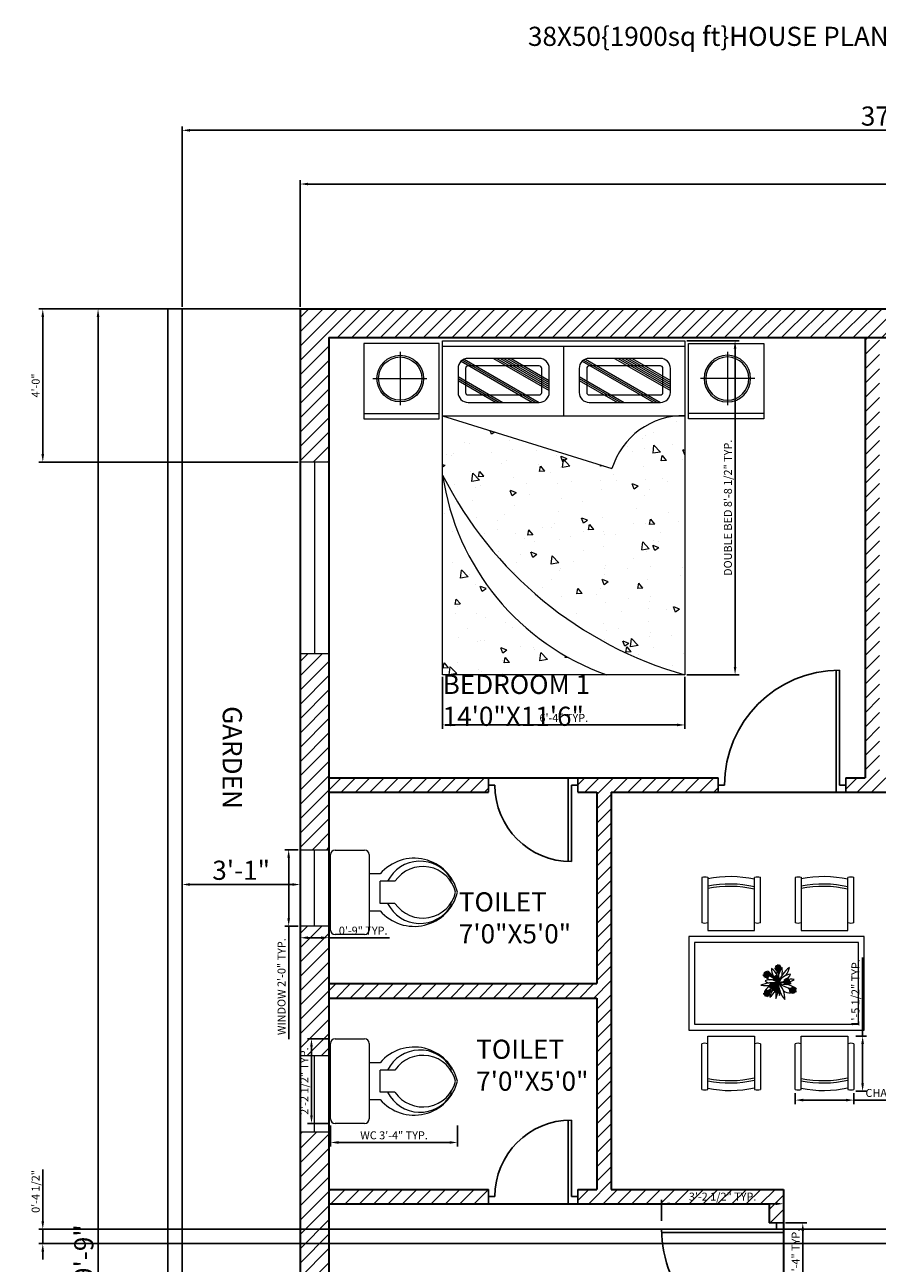
# Model space of a CAD drawing. Units: inches. Extents: x 3618 to 4156, y 1271 to 2023.
# Tile 4 of 5: x 3618 to 3886, y 1635 to 2023. Entities that reach past the tile are written whole.
import ezdxf

# ---------------------------------------------------------------- set-up
doc = ezdxf.new("R2010")
doc.units = ezdxf.units.IN
for name, color, linetype, lineweight in [('A-ANNO-DIMS', 2, 'Continuous', 18), ('A-ANNO-TITL', 7, 'Continuous', 25), ('A-AREA-IDEN', 7, 'Continuous', 18), ('A-DOOR', 4, 'Continuous', 25), ('A-FLOR-FIXT', 9, 'Continuous', 18), ('A-FURN', 8, 'Continuous', 18), ('A-FURN-PATT', 9, 'Continuous', 13), ('A-GLAZ', 4, 'Continuous', 18), ('A-WALL', 7, 'Continuous', 35), ('A-WALL-PATT', 252, 'Continuous', 13), ('C-PROP', 7, 'Continuous', 25)]:
    doc.layers.add(name, color=color, linetype=linetype, lineweight=lineweight)
doc.styles.get("Standard").update_dxf_attribs({"font": 'arial.ttf'})
doc.dimstyles.new('ISO-25', dxfattribs={"dimtxt": 2.5, "dimasz": 2.5, "dimexe": 1.25, "dimexo": 0.625, "dimtad": 1, "dimdec": 0, "dimlunit": 3, "dimtxsty": 'Standard', "dimcen": 2.5, "dimadec": 0, "dimazin": 0, "dimtfac": 1, "dimtdec": 0, "dimtmove": 0, "dimatfit": 3, "dimfxl": 1, "dimarcsym": 0})

# ---------------------------------------------------------------- blocks, each defined once
blk = doc.blocks.new('*D3')
at = {"layer": 'A-ANNO-DIMS', "color": 0, "lineweight": -2, "transparency": 16777216}
for p, q in [((3667.69, 1768.79), (3667.69, 1752.14)), ((3704.69, 1768.79), (3704.69, 1752.14)), ((3702.19, 1753.39), (3670.19, 1753.39))]:
    blk.add_line(p, q, dxfattribs=at)
at = {"layer": 'A-ANNO-DIMS', "color": 0, "transparency": 16777216}
for points in [[(3670.19, 1753.81), (3670.19, 1752.97), (3667.69, 1753.39)], [(3702.19, 1753.81), (3702.19, 1752.97), (3704.69, 1753.39)]]:
    blk.add_solid(points, dxfattribs=at)
at = {"layer": 'Defpoints', "color": 0, "transparency": 16777216}
for p in [(3667.69, 1769.42), (3704.69, 1769.42), (3667.69, 1753.39)]:
    blk.add_point(p, dxfattribs=at)
at = {"layer": 'A-ANNO-DIMS', "color": 0, "transparency": 16777216, "insert": (3686.19, 1757.08), "char_height": 6, "attachment_point": 5}
blk.add_mtext('3\'-1"', dxfattribs=at)
blk = doc.blocks.new('*D4')
at = {"layer": 'A-ANNO-DIMS', "color": 0, "lineweight": -2, "transparency": 16777216}
for p, q in [((3667.69, 1934.44), (3667.69, 1991.05)), ((3670.19, 1989.8), (4113.19, 1989.8)), ((4115.69, 1934.44), (4115.69, 1991.05))]:
    blk.add_line(p, q, dxfattribs=at)
at = {"layer": 'A-ANNO-DIMS', "color": 0, "transparency": 16777216}
for points in [[(3670.19, 1990.21), (3670.19, 1989.38), (3667.69, 1989.8)], [(4113.19, 1990.21), (4113.19, 1989.38), (4115.69, 1989.8)]]:
    blk.add_solid(points, dxfattribs=at)
at = {"layer": 'Defpoints', "color": 0, "transparency": 16777216}
for p in [(4115.69, 1989.8), (3667.69, 1933.81), (4115.69, 1933.81)]:
    blk.add_point(p, dxfattribs=at)
at = {"layer": 'A-ANNO-DIMS', "color": 0, "transparency": 16777216, "insert": (3891.69, 1993.49), "char_height": 6, "width": 8.5863, "attachment_point": 5}
blk.add_mtext('37\'-4"', dxfattribs=at)
blk = doc.blocks.new('*D8')
at = {"layer": 'A-ANNO-DIMS', "color": 0, "lineweight": -2, "transparency": 16777216}
for p, q in [((3662.56, 1933.81), (3640.11, 1933.81)), ((3641.36, 1931.31), (3641.36, 1339.81)), ((3662.56, 1337.31), (3640.11, 1337.31))]:
    blk.add_line(p, q, dxfattribs=at)
at = {"layer": 'A-ANNO-DIMS', "color": 0, "transparency": 16777216}
for points in [[(3640.94, 1931.31), (3641.77, 1931.31), (3641.36, 1933.81)], [(3640.94, 1339.81), (3641.77, 1339.81), (3641.36, 1337.31)]]:
    blk.add_solid(points, dxfattribs=at)
at = {"layer": 'Defpoints', "color": 0, "transparency": 16777216}
for p in [(3663.19, 1933.81), (3641.36, 1337.31), (3663.19, 1337.31)]:
    blk.add_point(p, dxfattribs=at)
at = {"layer": 'A-ANNO-DIMS', "color": 0, "transparency": 16777216, "insert": (3637.67, 1635.56), "char_height": 6, "attachment_point": 5, "rotation": 90}
blk.add_mtext('49\'-9"', dxfattribs=at)
blk = doc.blocks.new('A$C02F3725D')
for p, q in [((0.025, 0.69), (0.435, 0.69)), ((0, 0.505), (0, 0.665)), ((0.46, 0.665), (0.46, 0.505)), ((0.435, 0.48), (0.025, 0.48)), ((0.13, 0.48), (0.13, 0.42)), ((0.33, 0.42), (0.33, 0.48)), ((0.17, 0.34), (0.17, 0.42)), ((0.17, 0.42), (0.29, 0.42)), ((0.29, 0.34), (0.29, 0.42)), ((0.1578, 0.035), (0.1724, 0.035)), ((0.2876, 0.035), (0.3022, 0.035))]:
    blk.add_line(p, q)
for centre, radius, start, end in [((0.025, 0.665), 0.025, 90, 180), ((0.435, 0.665), 0.025, 0, 90), ((0.025, 0.505), 0.025, 180, 270), ((0.435, 0.505), 0.025, 270, 0), ((0.2874, 0.2356), 0.2425, 130.48854, 256.29645), ((0.1726, 0.2356), 0.2425, 283.70355, 49.51146), ((0.2568, 0.2042), 0.196, 116.27421, 239.66679), ((0.2732, 0.1883), 0.1834, 124.2157, 256.39399), ((0.1868, 0.1883), 0.1834, 283.60601, 55.7843), ((0.2032, 0.2042), 0.196, 300.33321, 63.72579)]:
    blk.add_arc(centre, radius, start, end)
blk = doc.blocks.new('DOOR-SWING-36')
for p, q in [((-1, -2.25), (-1, 36)), ((0, 0), (0, 36)), ((-38, 0), (-38, 2.25)), ((-36, 0), (-38, 0)), ((-38, 0), (-38, -2.25)), ((2, 0), (0, 0)), ((2, 2.25), (2, -2.25))]:
    blk.add_line(p, q)
blk.add_arc((0, 0), 36, 90, 180)
blk = doc.blocks.new('DOOR-SWING-24')
for p, q in [((-26, 0), (-26, 2.25)), ((-1, 2.25), (-1, -24)), ((2, -2.25), (2, 2.25)), ((-24, 0), (-26, 0)), ((-26, 0), (-26, -2.25)), ((2, 0), (0, 0)), ((0, 0), (0, -24))]:
    blk.add_line(p, q)
blk.add_arc((0, 0), 24, 180, 270)
blk = doc.blocks.new('WINDOW-24X9')
for p, q in [((0, 0), (0, 9)), ((0, 9), (24, 9)), ((24, 9), (24, 0)), ((24, 4.5), (0, 4.5)), ((24, 0), (0, 0))]:
    blk.add_line(p, q)
blk = doc.blocks.new('WINDOW-60X9')
for p, q in [((0, 60), (0, 0)), ((9, 60), (0, 60)), ((4.5, 60), (4.5, 0)), ((9, 0), (9, 60)), ((0, 0), (9, 0))]:
    blk.add_line(p, q)
blk = doc.blocks.new('CHAIR-DINING')
for p, q in [((1.87, 0.3), (1.87, 17.03)), ((1.87, 17.03), (16.54, 17.03)), ((16.54, 17.03), (16.54, 0.33)), ((0.04, 0.33), (0.04, 14.61)), ((18.37, 14.63), (18.37, 0.3))]:
    blk.add_line(p, q)
for centre, radius, start, end in [((0.96, 11.91), 2.86, 72.2774, 109.7376), ((17.51, 11.91), 2.86, 72.2774, 109.7376), ((8.76, 36.58), 33.52, 258.1438, 283.4274), ((0.99, 3.02), 2.86, 250.4535, 287.9116), ((8.76, 36.58), 34.25, 258.4012, 283.1346), ((8.76, 36.08), 36.09, 258.9982, 282.4562), ((17.5, 3.02), 2.86, 250.2624, 287.7226)]:
    blk.add_arc(centre, radius, start, end)
blk = doc.blocks.new('NIGHTSTAND-24')
for p, q in [((0, 23.56), (0, 0)), ((23.56, 23.56), (0, 23.56)), ((23.56, 0), (23.56, 23.56)), ((11.4, 20.97), (11.4, 4.24)), ((2.83, 12.61), (19.77, 12.61)), ((0, 1.65), (23.56, 1.65)), ((0, 0), (23.56, 0))]:
    blk.add_line(p, q)
for radius in [7.3, 6.77]:
    blk.add_circle((11.4, 12.61), radius)
blk = doc.blocks.new('BED-DOUBLE')
for p, q in [((0, 0), (0, 104.72)), ((0, 104.72), (75.92, 104.72)), ((0, 103.01), (75.92, 103.01)), ((37.96, 81.21), (37.96, 103.01)), ((75.92, 104.72), (75.92, 0)), ((0, 81.21), (53.06, 64.63)), ((0, 81.21), (75.92, 81.21)), ((75.92, 0), (0, 0))]:
    blk.add_line(p, q)
for centre, radius, start, end in [((75.45, 57.8), 23.41, 88.8468, 163.0453), ((109.27, 117.79), 122.42, 206.7955, 254.1914), ((77.5, 73.85), 78.32, 188.2583, 250.5572)]:
    blk.add_arc(centre, radius, start, end)
blk = doc.blocks.new('FLOWER-TABLE-ARRANGEMENT-BLOOM')
for centre, radius, start, end in [((0.82, -1.12), 2.18, 82.3009, 112.0255), ((0.29, 3.07), 2.18, 262.3009, 279.7139), ((1.21, 2.21), 1.17, 214.9663, 235.8146), ((0.15, 0.37), 1.17, 61.3074, 85.3856), ((1.2, -0.14), 1.18, 94.4763, 143.7634), ((0.16, 1.74), 1.18, 274.4763, 295.3557), ((0.59, 0.46), 0.778, 48.0547, 114.4672), ((0.79, 1.75), 0.778, 228.0547, 246.7161), ((2.72, 3.24), 2.72, 212.0897, 233.7438), ((-1.2, -0.41), 2.72, 32.0897, 53.7438), ((2.16, -0.69), 2.02, 121.2895, 147.5521), ((-0.59, 2.13), 2.02, 301.2895, 327.5521), ((-0.34, 1.33), 1.48, 307.8084, 348.7946), ((2.02, -0.13), 1.48, 150.6073, 168.7946), ((1.8, 1.93), 1.12, 178.5956, 203.6124), ((-0.01, 1.07), 1.12, 23.4487, 52.2657), ((2.9, 0.22), 1.97, 155.3732, 184.4609), ((-0.85, 0.89), 1.97, 335.3732, 4.4609), ((3.7, 1.79), 2.7, 172.5374, 196.1531), ((-1.57, 1.39), 2.7, 352.5374, 16.1531), ((2.46, 0.77), 1.38, 168.4621, 201.5435), ((2.78, 0.58), 1.74, 124.2737, 164.5097), ((1.02, 1.97), 0.934, 275.896, 336.1019), ((1.96, 0.66), 0.934, 95.896, 156.1019), ((1.46, -0.09), 1.19, 68.5561, 107.2542), ((0.03, 0.02), 1.48, 359.1564, 43.4376), ((2.59, 1.02), 1.48, 179.1564, 223.4376), ((1.54, 2.15), 1.19, 248.5561, 287.2542), ((2.28, 2.7), 2.03, 234.6665, 268.9653), ((2.27, 1.28), 1.18, 142.4708, 164.9809), ((-0.17, 0.54), 1.38, 348.4621, 358.2981), ((0.17, 1.76), 1.18, 348.7129, 11.758), ((1.83, 1.15), 0.732, 235.6133, 272.6537), ((0.13, 2.48), 1.74, 326.3124, 344.5097), ((1.87, -0.07), 1.35, 80.7415, 101.1747), ((1.07, -0.99), 2.03, 54.6665, 73.9559), ((1.33, 2.37), 1.35, 285.5442, 304.4617), ((1.14, 0.31), 0.732, 8.5521, 36.3024)]:
    blk.add_arc(centre, radius, start, end)
blk = doc.blocks.new('*D26')
at = {"layer": 'A-ANNO-DIMS', "color": 0, "lineweight": -2, "transparency": 16777216}
for p, q in [((3859.81, 1687.94), (3859.81, 1684.56)), ((3862.31, 1685.81), (3875.68, 1685.81)), ((3878.18, 1687.94), (3878.18, 1684.56)), ((3878.18, 1685.81), (3914.8, 1685.81))]:
    blk.add_line(p, q, dxfattribs=at)
at = {"layer": 'A-ANNO-DIMS', "color": 0, "transparency": 16777216}
for points in [[(3862.31, 1686.23), (3862.31, 1685.39), (3859.81, 1685.81)], [(3875.68, 1686.23), (3875.68, 1685.39), (3878.18, 1685.81)]]:
    blk.add_solid(points, dxfattribs=at)
at = {"layer": 'Defpoints', "color": 0, "transparency": 16777216}
for p in [(3859.81, 1688.57), (3878.18, 1688.57), (3878.18, 1685.81)]:
    blk.add_point(p, dxfattribs=at)
at = {"layer": 'A-ANNO-DIMS', "color": 0, "transparency": 16777216, "insert": (3897.74, 1687.73), "char_height": 2.5, "attachment_point": 5}
blk.add_mtext('CHAIR 1\'-6 1/2" TYP.', dxfattribs=at)
blk = doc.blocks.new('*D27')
at = {"layer": 'A-ANNO-DIMS', "color": 0, "lineweight": -2, "transparency": 16777216}
for p, q in [((3880.94, 1705.88), (3880.94, 1730.46)), ((3878.81, 1705.88), (3882.19, 1705.88)), ((3880.94, 1691.07), (3880.94, 1703.38)), ((3878.81, 1688.57), (3882.19, 1688.57))]:
    blk.add_line(p, q, dxfattribs=at)
at = {"layer": 'A-ANNO-DIMS', "color": 0, "transparency": 16777216}
for points in [[(3880.52, 1703.38), (3881.35, 1703.38), (3880.94, 1705.88)], [(3880.52, 1691.07), (3881.35, 1691.07), (3880.94, 1688.57)]]:
    blk.add_solid(points, dxfattribs=at)
at = {"layer": 'Defpoints', "color": 0, "transparency": 16777216}
for p in [(3878.18, 1705.88), (3880.94, 1705.88), (3878.18, 1688.57)]:
    blk.add_point(p, dxfattribs=at)
at = {"layer": 'A-ANNO-DIMS', "color": 0, "transparency": 16777216, "insert": (3879.02, 1719.42), "char_height": 2.5, "attachment_point": 5, "rotation": 90}
blk.add_mtext('1\'-5 1/2" TYP.', dxfattribs=at)
blk = doc.blocks.new('*D30')
at = {"layer": 'A-ANNO-DIMS', "color": 0, "lineweight": -2, "transparency": 16777216}
for p, q in [((3714.2, 1677.87), (3714.2, 1671.28)), ((3753.99, 1677.87), (3753.99, 1671.28)), ((3751.49, 1672.53), (3716.7, 1672.53))]:
    blk.add_line(p, q, dxfattribs=at)
at = {"layer": 'A-ANNO-DIMS', "color": 0, "transparency": 16777216}
for points in [[(3716.7, 1672.94), (3716.7, 1672.11), (3714.2, 1672.53)], [(3751.49, 1672.94), (3751.49, 1672.11), (3753.99, 1672.53)]]:
    blk.add_solid(points, dxfattribs=at)
at = {"layer": 'Defpoints', "color": 0, "transparency": 16777216}
for p in [(3714.2, 1678.5), (3753.99, 1678.5), (3714.2, 1672.53)]:
    blk.add_point(p, dxfattribs=at)
at = {"layer": 'A-ANNO-DIMS', "color": 0, "transparency": 16777216, "insert": (3734.1, 1674.45), "char_height": 2.5, "attachment_point": 5}
blk.add_mtext('WC 3\'-4" TYP.', dxfattribs=at)
blk = doc.blocks.new('*D31')
at = {"layer": 'A-ANNO-DIMS', "color": 0, "lineweight": -2, "transparency": 16777216}
for p, q in [((3713.58, 1705.02), (3706.99, 1705.02)), ((3708.24, 1681), (3708.24, 1702.52)), ((3713.58, 1678.5), (3706.99, 1678.5))]:
    blk.add_line(p, q, dxfattribs=at)
at = {"layer": 'A-ANNO-DIMS', "color": 0, "transparency": 16777216}
for points in [[(3707.82, 1702.52), (3708.65, 1702.52), (3708.24, 1705.02)], [(3707.82, 1681), (3708.65, 1681), (3708.24, 1678.5)]]:
    blk.add_solid(points, dxfattribs=at)
at = {"layer": 'Defpoints', "color": 0, "transparency": 16777216}
for p in [(3708.24, 1705.02), (3714.2, 1705.02), (3714.2, 1678.5)]:
    blk.add_point(p, dxfattribs=at)
at = {"layer": 'A-ANNO-DIMS', "color": 0, "transparency": 16777216, "insert": (3706.32, 1691.76), "char_height": 2.5, "attachment_point": 5, "rotation": 90}
blk.add_mtext('2\'-2 1/2" TYP.', dxfattribs=at)
blk = doc.blocks.new('*D32')
at = {"layer": 'A-ANNO-DIMS', "color": 0, "lineweight": -2, "transparency": 16777216}
for p, q in [((3856.81, 1647.31), (3863.44, 1647.31)), ((3862.19, 1609.81), (3862.19, 1644.81)), ((3856.81, 1607.31), (3863.44, 1607.31))]:
    blk.add_line(p, q, dxfattribs=at)
at = {"layer": 'A-ANNO-DIMS', "color": 0, "transparency": 16777216}
for points in [[(3861.77, 1644.81), (3862.6, 1644.81), (3862.19, 1647.31)], [(3861.77, 1609.81), (3862.6, 1609.81), (3862.19, 1607.31)]]:
    blk.add_solid(points, dxfattribs=at)
at = {"layer": 'Defpoints', "color": 0, "transparency": 16777216}
for p in [(3856.19, 1647.31), (3862.19, 1647.31), (3856.19, 1607.31)]:
    blk.add_point(p, dxfattribs=at)
at = {"layer": 'A-ANNO-DIMS', "color": 0, "transparency": 16777216, "insert": (3860.27, 1627.31), "char_height": 2.5, "attachment_point": 5, "rotation": 90}
blk.add_mtext('ROOM DOOR 3\'-4" TYP.', dxfattribs=at)
blk = doc.blocks.new('*D33')
at = {"layer": 'A-ANNO-DIMS', "color": 0, "lineweight": -2, "transparency": 16777216}
for p, q in [((3817.94, 1647.94), (3817.94, 1654.56)), ((3856.19, 1647.94), (3856.19, 1654.56)), ((3853.69, 1653.31), (3820.44, 1653.31))]:
    blk.add_line(p, q, dxfattribs=at)
at = {"layer": 'A-ANNO-DIMS', "color": 0, "transparency": 16777216}
for points in [[(3820.44, 1653.73), (3820.44, 1652.89), (3817.94, 1653.31)], [(3853.69, 1653.73), (3853.69, 1652.89), (3856.19, 1653.31)]]:
    blk.add_solid(points, dxfattribs=at)
at = {"layer": 'Defpoints', "color": 0, "transparency": 16777216}
for p in [(3817.94, 1653.31), (3817.94, 1647.31), (3856.19, 1647.31)]:
    blk.add_point(p, dxfattribs=at)
at = {"layer": 'A-ANNO-DIMS', "color": 0, "transparency": 16777216, "insert": (3837.06, 1655.23), "char_height": 2.5, "attachment_point": 5}
blk.add_mtext('3\'-2 1/2" TYP.', dxfattribs=at)
blk = doc.blocks.new('*D36')
at = {"layer": 'A-ANNO-DIMS', "color": 0, "lineweight": -2, "transparency": 16777216}
for p, q in [((3704.06, 1764.31), (3699.84, 1764.31)), ((3701.09, 1761.81), (3701.09, 1742.81)), ((3704.06, 1740.31), (3699.84, 1740.31)), ((3701.09, 1740.31), (3701.09, 1704.92))]:
    blk.add_line(p, q, dxfattribs=at)
at = {"layer": 'A-ANNO-DIMS', "color": 0, "transparency": 16777216}
for points in [[(3700.67, 1761.81), (3701.5, 1761.81), (3701.09, 1764.31)], [(3700.67, 1742.81), (3701.5, 1742.81), (3701.09, 1740.31)]]:
    blk.add_solid(points, dxfattribs=at)
at = {"layer": 'Defpoints', "color": 0, "transparency": 16777216}
for p in [(3704.69, 1764.31), (3701.09, 1740.31), (3704.69, 1740.31)]:
    blk.add_point(p, dxfattribs=at)
at = {"layer": 'A-ANNO-DIMS', "color": 0, "transparency": 16777216, "insert": (3699.17, 1721.37), "char_height": 2.5, "attachment_point": 5, "rotation": 90}
blk.add_mtext('WINDOW 2\'-0" TYP.', dxfattribs=at)
blk = doc.blocks.new('*D37')
at = {"layer": 'A-ANNO-DIMS', "color": 0, "lineweight": -2, "transparency": 16777216}
for p, q in [((3704.69, 1739.69), (3704.69, 1735.46)), ((3713.69, 1739.69), (3713.69, 1735.46)), ((3707.19, 1736.71), (3711.19, 1736.71)), ((3713.69, 1736.71), (3732.68, 1736.71))]:
    blk.add_line(p, q, dxfattribs=at)
at = {"layer": 'A-ANNO-DIMS', "color": 0, "transparency": 16777216}
for points in [[(3707.19, 1737.13), (3707.19, 1736.29), (3704.69, 1736.71)], [(3711.19, 1737.13), (3711.19, 1736.29), (3713.69, 1736.71)]]:
    blk.add_solid(points, dxfattribs=at)
at = {"layer": 'Defpoints', "color": 0, "transparency": 16777216}
for p in [(3704.69, 1740.31), (3713.69, 1740.31), (3713.69, 1736.71)]:
    blk.add_point(p, dxfattribs=at)
at = {"layer": 'A-ANNO-DIMS', "color": 0, "transparency": 16777216, "insert": (3724.43, 1738.61), "char_height": 2.5, "attachment_point": 5}
blk.add_mtext('0\'-9" TYP.', dxfattribs=at)
blk = doc.blocks.new('*D44')
at = {"layer": 'A-ANNO-DIMS', "color": 0, "lineweight": -2, "transparency": 16777216}
for p, q in [((3825.88, 1923.84), (3842.22, 1923.84)), ((3840.97, 1821.62), (3840.97, 1921.34)), ((3825.88, 1819.12), (3842.22, 1819.12))]:
    blk.add_line(p, q, dxfattribs=at)
at = {"layer": 'A-ANNO-DIMS', "color": 0, "transparency": 16777216}
for points in [[(3840.55, 1921.34), (3841.38, 1921.34), (3840.97, 1923.84)], [(3840.55, 1821.62), (3841.38, 1821.62), (3840.97, 1819.12)]]:
    blk.add_solid(points, dxfattribs=at)
at = {"layer": 'Defpoints', "color": 0, "transparency": 16777216}
for p in [(3825.26, 1923.84), (3840.97, 1923.84), (3825.26, 1819.12)]:
    blk.add_point(p, dxfattribs=at)
at = {"layer": 'A-ANNO-DIMS', "color": 0, "transparency": 16777216, "insert": (3839.05, 1871.48), "char_height": 2.5, "attachment_point": 5, "rotation": 90}
blk.add_mtext('DOUBLE BED 8\'-8 1/2" TYP.', dxfattribs=at)
blk = doc.blocks.new('*D45')
at = {"layer": 'A-ANNO-DIMS', "color": 0, "lineweight": -2, "transparency": 16777216}
for p, q in [((3749.34, 1818.49), (3749.34, 1802.16)), ((3825.26, 1818.49), (3825.26, 1802.16)), ((3751.84, 1803.41), (3822.76, 1803.41))]:
    blk.add_line(p, q, dxfattribs=at)
at = {"layer": 'A-ANNO-DIMS', "color": 0, "transparency": 16777216}
for points in [[(3751.84, 1803.83), (3751.84, 1802.99), (3749.34, 1803.41)], [(3822.76, 1803.83), (3822.76, 1802.99), (3825.26, 1803.41)]]:
    blk.add_solid(points, dxfattribs=at)
at = {"layer": 'Defpoints', "color": 0, "transparency": 16777216}
for p in [(3749.34, 1819.12), (3825.26, 1819.12), (3825.26, 1803.41)]:
    blk.add_point(p, dxfattribs=at)
at = {"layer": 'A-ANNO-DIMS', "color": 0, "transparency": 16777216, "insert": (3787.3, 1805.31), "char_height": 2.5, "attachment_point": 5}
blk.add_mtext('6\'-4" TYP.', dxfattribs=at)
blk = doc.blocks.new('*D55')
at = {"layer": 'A-ANNO-DIMS', "color": 0, "lineweight": -2, "transparency": 16777216}
for p, q in [((3704.69, 1934.44), (3704.69, 1974.21)), ((3707.19, 1972.96), (4113.19, 1972.96)), ((4115.69, 1934.44), (4115.69, 1974.21))]:
    blk.add_line(p, q, dxfattribs=at)
at = {"layer": 'A-ANNO-DIMS', "color": 0, "transparency": 16777216}
for points in [[(3707.19, 1973.38), (3707.19, 1972.54), (3704.69, 1972.96)], [(4113.19, 1973.38), (4113.19, 1972.54), (4115.69, 1972.96)]]:
    blk.add_solid(points, dxfattribs=at)
at = {"layer": 'Defpoints', "color": 0, "transparency": 16777216}
for p in [(4115.69, 1972.96), (3704.69, 1933.81), (4115.69, 1933.81)]:
    blk.add_point(p, dxfattribs=at)
at = {"layer": 'A-ANNO-DIMS', "color": 0, "transparency": 16777216, "insert": (3910.19, 1974.86), "char_height": 2.5, "attachment_point": 5}
blk.add_mtext('34\'-3"', dxfattribs=at)
blk = doc.blocks.new('*D57')
at = {"layer": 'A-ANNO-DIMS', "color": 0, "lineweight": -2, "transparency": 16777216}
for p, q in [((3704.06, 1933.81), (3622.79, 1933.81)), ((3624.04, 1931.31), (3624.04, 1888.31)), ((3704.06, 1885.81), (3622.79, 1885.81))]:
    blk.add_line(p, q, dxfattribs=at)
at = {"layer": 'A-ANNO-DIMS', "color": 0, "transparency": 16777216}
for points in [[(3623.62, 1931.31), (3624.45, 1931.31), (3624.04, 1933.81)], [(3623.62, 1888.31), (3624.45, 1888.31), (3624.04, 1885.81)]]:
    blk.add_solid(points, dxfattribs=at)
at = {"layer": 'Defpoints', "color": 0, "transparency": 16777216}
for p in [(3704.69, 1933.81), (3624.04, 1885.81), (3704.69, 1885.81)]:
    blk.add_point(p, dxfattribs=at)
at = {"layer": 'A-ANNO-DIMS', "color": 0, "transparency": 16777216, "insert": (3622.14, 1909.81), "char_height": 2.5, "attachment_point": 5, "rotation": 90}
blk.add_mtext('4\'-0"', dxfattribs=at)
blk = doc.blocks.new('*D59')
at = {"layer": 'A-ANNO-DIMS', "color": 0, "lineweight": -2, "transparency": 16777216}
for p, q in [((3624.04, 1647.81), (3624.04, 1664.03)), ((3940.35, 1645.31), (3622.79, 1645.31)), ((3624.04, 1640.81), (3624.04, 1645.31)), ((3940.35, 1640.81), (3622.79, 1640.81)), ((3624.04, 1638.31), (3624.04, 1635.81))]:
    blk.add_line(p, q, dxfattribs=at)
at = {"layer": 'A-ANNO-DIMS', "color": 0, "transparency": 16777216}
for points in [[(3623.62, 1647.81), (3624.45, 1647.81), (3624.04, 1645.31)], [(3623.62, 1638.31), (3624.45, 1638.31), (3624.04, 1640.81)]]:
    blk.add_solid(points, dxfattribs=at)
at = {"layer": 'Defpoints', "color": 0, "transparency": 16777216}
for p in [(3624.04, 1645.31), (3940.98, 1645.31), (3940.98, 1640.81)]:
    blk.add_point(p, dxfattribs=at)
at = {"layer": 'A-ANNO-DIMS', "color": 0, "transparency": 16777216, "insert": (3622.12, 1657.17), "char_height": 2.5, "attachment_point": 5, "rotation": 90}
blk.add_mtext('0\'-4 1/2"', dxfattribs=at)

msp = doc.modelspace()

# ---------------------------------------------------------------- hatches: boundary and pattern name
at = {"layer": 'A-FURN-PATT'}
h = msp.add_hatch(dxfattribs=at)
h.set_pattern_fill('ANSI31', color=256, scale=0.16491505, angle=105.04163, style=0)
h.paths.add_polyline_path([(3756.24, 1918.14), (3756.08, 1918.07), (3755.89, 1917.99), (3755.71, 1917.89), (3755.54, 1917.78), (3755.38, 1917.67), (3755.23, 1917.54), (3755.08, 1917.4), (3755.02, 1917.33), (3777.27, 1904.51), (3779.59, 1904.51), (3779.81, 1904.51), (3779.87, 1904.52)])
h = msp.add_hatch(dxfattribs=at)
h.set_pattern_fill('ANSI31', color=256, scale=0.17286572, angle=105.04163, style=0)
h.paths.add_polyline_path([(3771.03, 1918.32), (3764.98, 1918.32), (3782.74, 1908.09), (3782.74, 1911.57)])
h = msp.add_hatch(dxfattribs=at)
h.set_pattern_fill('ANSI31', color=256, scale=0.16492001, angle=105.04163, style=0)
h.paths.add_polyline_path([(3794.2, 1918.14), (3794.04, 1918.07), (3793.85, 1917.99), (3793.68, 1917.89), (3793.51, 1917.78), (3793.34, 1917.67), (3793.19, 1917.54), (3793.04, 1917.4), (3792.98, 1917.33), (3815.23, 1904.51), (3817.56, 1904.51), (3817.66, 1904.51), (3817.76, 1904.51), (3817.83, 1904.52)])
h = msp.add_hatch(dxfattribs=at)
h.set_pattern_fill('ANSI31', color=256, scale=0.17288008, angle=105.04163, style=0)
h.paths.add_polyline_path([(3808.99, 1918.32), (3802.94, 1918.32), (3820.7, 1908.09), (3820.7, 1911.57)])
h = msp.add_hatch(dxfattribs=at)
h.set_pattern_fill('ANSI31', color=256, scale=0.16491844, angle=105.04163, style=0)
h.paths.add_polyline_path([(3754.16, 1912.77), (3754.16, 1911.26), (3765.88, 1904.51), (3768.5, 1904.51)])
h = msp.add_hatch(dxfattribs=at)
h.set_pattern_fill('ANSI31', color=256, scale=0.16492339, angle=105.04163, style=0)
h.paths.add_polyline_path([(3792.12, 1912.77), (3792.12, 1911.26), (3803.84, 1904.51), (3806.46, 1904.51)])
h = msp.add_hatch(dxfattribs=at)
h.set_pattern_fill('AR-CONC', color=256, scale=0.104721, angle=360, style=0)
h.set_pattern_definition([(130, (4719.83, -4019.08), (-19.07861, -1.66916), [1.99494, -21.94434]), (185, (4719.83, -4019.08), (3.690674, 20.007695), [1.59595, -17.555474]), (79.549, (4718.24, -4019.218), (-15.388006, 18.33844), [1.69544, -18.64981]), (133.8158, (4719.83, -4013.76), (-28.38774, -4.40273), [2.99241, -32.91651]), (83.3644, (4717.465, -4014.126), (-24.86127, 25.91072), [2.54316, -27.97472]), (188.816, (4719.83, -4013.76), (-24.86131, 25.91067), [2.39393, -26.33321]), (159, (4717.17, -4015.09), (-15.877303, -10.709375), [1.99494, -21.94434]), (214, (4717.17, -4015.09), (-6.47199, 19.2884), [1.59595, -17.555474]), (108.5486, (4715.847, -4015.982), (-22.349247, 8.579066), [1.69544, -18.64981]), (142.5, (4719.83, -4019.079), (-0.3234425, 8.8547114), [0, -17.34268, 0, -17.821467, 0, -17.621972]), (172.5, (4719.83, -4019.079), (-6.99744, 10.491037), [0, -10.160896, 0, -16.943693, 0, -6.716299]), (212.5, (4725.762, -4019.079), (-14.19922, -0.599921), [0, -6.6498, 0, -20.747379, 0, -27.530176]), (222.5, (4728.422, -4019.079), (-15.512277, 2.662695), [0, -8.64474, 0, -13.778388, 0, -19.550415])])
edge = h.paths.add_edge_path()
edge.add_ellipse((3824.79, 1876.92), major_axis=(16.55, -16.55), ratio=1, start_angle=136.1532, end_angle=208.0453, ccw=False)
edge.add_line((3824.32, 1900.33), (3825.26, 1900.33))
edge.add_line((3825.26, 1900.33), (3825.26, 1819.12))
edge.add_ellipse((3858.61, 1936.91), major_axis=(86.56, -86.56), ratio=1, start_angle=251.7955, end_angle=299.1914, ccw=False)
edge.add_line((3749.34, 1881.72), (3749.34, 1900.33))
edge.add_line((3749.34, 1900.33), (3802.39, 1883.75))
edge = h.paths.add_edge_path()
edge.add_line((3800.77, 1819.12), (3749.34, 1819.12))
edge.add_line((3749.34, 1819.12), (3749.34, 1881.72))
edge.add_ellipse((3826.84, 1892.97), major_axis=(-55.38, -55.38), ratio=1, start_angle=323.2583, end_angle=385.5572)
at = {"layer": 'A-WALL-PATT'}
h = msp.add_hatch(dxfattribs=at)
h.set_pattern_fill('ANSI31', color=256)
h.paths.add_polyline_path([(4115.69, 1933.81), (3704.69, 1933.81), (3704.69, 1885.81), (3713.69, 1885.81), (3713.69, 1924.81), (4115.69, 1924.81)])
h.paths.add_polyline_path([(3886.19, 1924.81), (3881.69, 1924.81), (3881.69, 1786.81), (3875.69, 1786.81), (3875.69, 1782.31), (3892.19, 1782.31), (3892.19, 1786.81), (3886.19, 1786.81)])
h.paths.add_polyline_path([(3763.69, 1784.56), (3763.69, 1786.81), (3713.69, 1786.81), (3713.69, 1782.31), (3763.69, 1782.31)], flags=17)
h.paths.add_polyline_path([(3713.69, 1825.81), (3704.69, 1825.81), (3704.69, 1764.31), (3713.69, 1764.31)])
h.paths.add_polyline_path([(3802.19, 1782.31), (3835.69, 1782.31), (3835.69, 1784.56), (3835.69, 1786.81), (3791.69, 1786.81), (3791.69, 1782.31), (3797.69, 1782.31), (3797.69, 1722.31), (3713.69, 1722.31), (3713.69, 1717.81), (3797.69, 1717.81), (3797.69, 1657.81), (3791.69, 1657.81), (3791.69, 1653.31), (3851.69, 1653.31), (3851.69, 1647.31), (3856.19, 1647.31), (3856.19, 1657.81), (3802.19, 1657.81)])
h.paths.add_polyline_path([(3713.69, 1740.31), (3704.69, 1740.31), (3704.69, 1699.81), (3713.69, 1699.81)])
h.paths.add_polyline_path([(3713.69, 1675.81), (3704.69, 1675.81), (3704.69, 1623.31), (3713.69, 1623.31)])
h.paths.add_polyline_path([(3743.18, 1533.31), (3713.69, 1533.31), (3713.69, 1563.31), (3704.69, 1563.31), (3704.69, 1524.31), (3743.18, 1524.31)])
h.paths.add_polyline_path([(3856.19, 1533.31), (3803.18, 1533.31), (3803.18, 1524.31), (3847.19, 1524.31), (3847.19, 1518.31), (3856.19, 1518.31)])
h.paths.add_polyline_path([(3856.19, 1607.31), (3853.94, 1607.31), (3851.69, 1607.31), (3851.69, 1533.31), (3856.19, 1533.31)])
h.paths.add_polyline_path([(3763.69, 1655.56), (3763.69, 1657.81), (3713.69, 1657.81), (3713.69, 1653.31), (3763.69, 1653.31)], flags=17)
h.paths.add_polyline_path([(4063.19, 1670.56), (4054.19, 1670.56), (4054.19, 1645.31), (3940.98, 1645.31), (3940.98, 1640.81), (4054.19, 1640.81), (4054.19, 1592.81), (4063.19, 1592.81)])
h.paths.add_polyline_path([(4063.19, 1532.81), (4054.19, 1532.81), (4054.19, 1454.31), (4063.19, 1454.31)])
h.paths.add_polyline_path([(4054.19, 1484.81), (3985.19, 1484.81), (3985.19, 1475.81), (4054.19, 1475.81)])
h.paths.add_polyline_path([(3925.19, 1484.81), (3856.19, 1484.81), (3856.19, 1490.81), (3847.19, 1490.81), (3847.19, 1475.81), (3925.19, 1475.81)])
h.paths.add_polyline_path([(4063.19, 1396.81), (3928.19, 1396.81), (3928.19, 1387.81), (4063.19, 1387.81)])
h.paths.add_polyline_path([(4063.19, 1418.31), (4054.19, 1418.31), (4054.19, 1396.81), (4063.19, 1396.81)])
h.paths.add_polyline_path([(4063.19, 1790.42), (4054.19, 1790.42), (4054.19, 1786.81), (3932.19, 1786.81), (3932.19, 1784.56), (3932.19, 1782.31), (4054.19, 1782.31), (4054.19, 1771.81), (4063.19, 1771.81)])
h.paths.add_polyline_path([(4070.69, 1840.81), (4058.69, 1840.81), (4058.69, 1890.81), (4056.44, 1890.81), (4054.19, 1890.81), (4054.19, 1826.42), (4063.19, 1826.42), (4063.19, 1831.81), (4070.69, 1831.81)])
h.paths.add_polyline_path([(4115.69, 1924.81), (4106.69, 1924.81), (4106.69, 1840.81), (4094.69, 1840.81), (4094.69, 1831.81), (4115.69, 1831.81)])
h.paths.add_polyline_path([(4063.19, 1731.81), (4058.69, 1731.81), (4054.19, 1731.81), (4054.19, 1706.56), (4063.19, 1706.56)])

# ---------------------------------------------------------------- linework, layer by layer
at = {"layer": 'A-FURN'}
for points in [[(3779.59, 1918.32), (3757.3, 1918.32, 0.414214), (3754.16, 1915.18), (3754.16, 1907.65, 0.414214), (3757.3, 1904.51), (3779.59, 1904.51, 0.414214), (3782.74, 1907.65), (3782.74, 1915.18, 0.414214)], [(3817.56, 1918.32), (3795.26, 1918.32, 0.414214), (3792.12, 1915.18), (3792.12, 1907.65, 0.414214), (3795.26, 1904.51), (3817.56, 1904.51, 0.414214), (3820.7, 1907.65), (3820.7, 1915.18, 0.414214)], [(3779.59, 1915.96), (3757.3, 1915.96, 0.414214), (3756.51, 1915.18), (3756.51, 1907.65, 0.414214), (3757.3, 1906.86), (3779.59, 1906.86, 0.414214), (3780.38, 1907.65), (3780.38, 1915.18, 0.414214)], [(3817.56, 1915.96), (3795.26, 1915.96, 0.414214), (3794.48, 1915.18), (3794.48, 1907.65, 0.414214), (3795.26, 1906.86), (3817.56, 1906.86, 0.414214), (3818.34, 1907.65), (3818.34, 1915.18, 0.414214)]]:
    msp.add_lwpolyline(points, format="xyb", close=True, dxfattribs=at)
for points in [[(3826.46, 1737.08), (3826.46, 1707.74), (3881.47, 1707.74), (3881.47, 1737.08)], [(3828.29, 1735.25), (3828.29, 1709.57), (3879.64, 1709.57), (3879.64, 1735.25)]]:
    msp.add_lwpolyline(points, close=True, dxfattribs=at)
for centre, radius, start, end in [((3867.55, 1726.28), 13.5, 172.5374, 196.1531), ((3841.19, 1724.27), 13.5, 352.5374, 16.1531), ((3849.79, 1719.17), 5.84, 61.3074, 85.3856), ((3855.05, 1728.34), 5.84, 214.9663, 235.8146), ((3843.04, 1715.28), 13.62, 32.0897, 53.7438), ((3862.64, 1733.51), 13.62, 212.0897, 233.7438), ((3848.97, 1722.66), 5.61, 23.4487, 52.2657), ((3858.01, 1726.96), 5.61, 178.5956, 203.6124), ((3862.94, 1720.2), 8.68, 124.2737, 164.5097), ((3854.1, 1727.16), 4.67, 275.896, 336.1019), ((3858.85, 1720.63), 4.67, 95.896, 156.1019), ((3860.38, 1723.73), 5.92, 142.4708, 164.9809), ((3849.88, 1726.13), 5.92, 348.7129, 11.758), ((3854.85, 1721.49), 2.72, 32.0897, 53.7438), ((3858.77, 1725.14), 2.72, 212.0897, 233.7438), ((3856.03, 1722.97), 1.12, 23.4487, 52.2657), ((3857.84, 1723.83), 1.12, 178.5956, 203.6124), ((3849.69, 1729.69), 8.68, 326.3124, 344.5097), ((3859.75, 1723.69), 2.7, 172.5374, 196.1531), ((3854.48, 1723.29), 2.7, 352.5374, 16.1531), ((3858.39, 1716.97), 6.73, 80.7415, 101.1747), ((3858.83, 1722.48), 1.74, 124.2737, 164.5097), ((3858.32, 1723.18), 1.18, 142.4708, 164.9809), ((3856.22, 1723.66), 1.18, 348.7129, 11.758), ((3856.18, 1724.38), 1.74, 326.3124, 344.5097), ((3853.12, 1711.7), 10.91, 82.3009, 112.0255), ((3850.49, 1732.64), 10.91, 262.3009, 279.7139), ((3855.04, 1716.61), 5.92, 94.4763, 143.7634), ((3849.8, 1726.02), 5.92, 274.4763, 295.3557), ((3851.98, 1719.63), 3.89, 48.0547, 114.4672), ((3852.97, 1726.06), 3.89, 228.0547, 246.7161), ((3859.83, 1713.88), 10.11, 121.2895, 147.5521), ((3846.05, 1727.94), 10.11, 301.2895, 327.5521), ((3847.3, 1723.96), 7.42, 307.8084, 348.7946), ((3859.13, 1716.66), 7.42, 150.6073, 168.7946), ((3863.53, 1718.42), 9.84, 155.3732, 184.4609), ((3844.77, 1721.75), 9.84, 335.3732, 4.4609), ((3861.32, 1721.14), 6.88, 168.4621, 201.5435), ((3856.34, 1716.86), 5.93, 68.5561, 107.2542), ((3856.75, 1728.04), 5.93, 248.5561, 287.2542), ((3860.44, 1730.79), 10.14, 234.6665, 268.9653), ((3849.19, 1717.42), 7.42, 359.1564, 43.4376), ((3862, 1722.41), 7.42, 179.1564, 223.4376), ((3848.18, 1719.99), 6.88, 348.4621, 358.2981), ((3856.86, 1720.78), 2.18, 82.3009, 112.0255), ((3856.34, 1724.96), 2.18, 262.3009, 279.7139), ((3858.2, 1723.06), 3.66, 235.6133, 272.6537), ((3857.25, 1724.11), 1.17, 214.9663, 235.8146), ((3856.2, 1722.27), 1.17, 61.3074, 85.3856), ((3857.25, 1721.76), 1.18, 94.4763, 143.7634), ((3856.2, 1723.64), 1.18, 274.4763, 295.3557), ((3856.64, 1722.36), 0.778, 48.0547, 114.4672), ((3856.83, 1723.65), 0.778, 228.0547, 246.7161), ((3855.45, 1724.03), 2.02, 301.2895, 327.5521), ((3858.21, 1721.21), 2.02, 121.2895, 147.5521), ((3855.7, 1723.23), 1.48, 307.8084, 348.7946), ((3858.07, 1721.77), 1.48, 150.6073, 168.7946), ((3855.19, 1722.79), 1.97, 335.3732, 4.4609), ((3858.94, 1722.12), 1.97, 155.3732, 184.4609), ((3858.5, 1722.67), 1.38, 168.4621, 201.5435), ((3857.06, 1723.87), 0.934, 275.896, 336.1019), ((3858.01, 1722.56), 0.934, 95.896, 156.1019), ((3857.51, 1721.81), 1.19, 68.5561, 107.2542), ((3858.64, 1722.92), 1.48, 179.1564, 223.4376), ((3857.59, 1724.05), 1.19, 248.5561, 287.2542), ((3858.33, 1724.6), 2.03, 234.6665, 268.9653), ((3856.08, 1721.92), 1.48, 359.1564, 43.4376), ((3854.4, 1712.38), 10.14, 54.6665, 73.9559), ((3855.88, 1722.44), 1.38, 348.4621, 358.2981), ((3855.66, 1729.16), 6.73, 285.5442, 304.4617), ((3857.88, 1723.05), 0.732, 235.6133, 272.6537), ((3857.92, 1721.83), 1.35, 80.7415, 101.1747), ((3857.12, 1720.91), 2.03, 54.6665, 73.9559), ((3854.75, 1718.86), 3.66, 8.5521, 36.3024), ((3857.37, 1724.27), 1.35, 285.5442, 304.4617), ((3857.19, 1722.21), 0.732, 8.5521, 36.3024)]:
    msp.add_arc(centre, radius, start, end, dxfattribs=at)
at = {"layer": 'A-WALL'}
for p, q in [((3704.69, 1933.81), (3704.69, 1524.31)), ((3704.69, 1933.81), (4115.69, 1933.81)), ((3713.69, 1924.81), (4115.69, 1924.81)), ((3713.69, 1924.81), (3713.69, 1533.31)), ((3881.69, 1924.81), (3881.69, 1786.81)), ((3713.69, 1786.81), (3835.69, 1786.81)), ((3875.69, 1786.81), (3881.69, 1786.81)), ((3713.69, 1782.31), (3763.69, 1782.31)), ((3791.69, 1782.31), (3797.69, 1782.31)), ((3797.69, 1782.31), (3797.69, 1722.31)), ((3802.19, 1782.31), (3802.19, 1657.81)), ((3802.19, 1782.31), (4054.19, 1782.31)), ((3713.69, 1722.31), (3797.69, 1722.31)), ((3713.69, 1717.81), (3797.69, 1717.81)), ((3797.69, 1717.81), (3797.69, 1657.81)), ((3713.69, 1657.81), (3763.69, 1657.81)), ((3791.69, 1657.81), (3797.69, 1657.81)), ((3802.19, 1657.81), (3856.19, 1657.81)), ((3856.19, 1657.81), (3856.19, 1518.31)), ((3713.69, 1653.31), (3851.69, 1653.31)), ((3851.69, 1653.31), (3851.69, 1647.31))]:
    msp.add_line(p, q, dxfattribs=at)
at = {"layer": 'C-PROP'}
for p, q in [((3663.19, 1933.81), (3663.19, 1524.31)), ((3663.19, 1933.81), (3667.69, 1933.81)), ((3667.69, 1933.81), (3667.69, 1524.31)), ((3667.69, 1933.81), (3704.69, 1933.81))]:
    msp.add_line(p, q, dxfattribs=at)

# ---------------------------------------------------------------- block references
at = {"layer": 'A-DOOR'}
for name, p in [('DOOR-SWING-36', (3873.69, 1784.56)), ('DOOR-SWING-24', (3789.69, 1784.56))]:
    msp.add_blockref(name, p, dxfattribs=at)
at = {"layer": 'A-DOOR', "extrusion": (0, 0, -1), "zscale": -1, "rotation": 180}
msp.add_blockref('DOOR-SWING-24', (-3789.69, 1655.56), dxfattribs=at)
at = {"layer": 'A-DOOR', "rotation": 90.00000000000087}
msp.add_blockref('DOOR-SWING-36', (3853.94, 1645.31), dxfattribs=at)
at = {"layer": 'A-FLOR-FIXT', "xscale": 57.66831845044013, "yscale": 57.66831845044013, "zscale": 57.66831845044013, "rotation": 90}
for p in [(3753.99, 1737.68), (3753.99, 1678.5)]:
    msp.add_blockref('A$C02F3725D', p, dxfattribs=at)
at = {"layer": 'A-FURN'}
for name, p in [('NIGHTSTAND-24', (3724.64, 1899.37)), ('BED-DOUBLE', (3749.34, 1819.12)), ('FLOWER-TABLE-ARRANGEMENT-BLOOM', (3853.33, 1726.17)), ('FLOWER-TABLE-ARRANGEMENT-BLOOM', (3849.69, 1724.04)), ('FLOWER-TABLE-ARRANGEMENT-BLOOM', (3852.85, 1722.87)), ('FLOWER-TABLE-ARRANGEMENT-BLOOM', (3849.79, 1718.21)), ('FLOWER-TABLE-ARRANGEMENT-BLOOM', (3851.52, 1720.54)), ('FLOWER-TABLE-ARRANGEMENT-BLOOM', (3852.94, 1719.37)), ('FLOWER-TABLE-ARRANGEMENT-BLOOM', (3857.94, 1719.18)), ('CHAIR-DINING', (3830.54, 1688.85)), ('CHAIR-DINING', (3859.81, 1688.85))]:
    msp.add_blockref(name, p, dxfattribs=at)
at = {"layer": 'A-FURN', "extrusion": (0, 0, -1), "zscale": -1}
msp.add_blockref('NIGHTSTAND-24', (-3849.95, 1899.37), dxfattribs=at)
at = {"layer": 'A-FURN', "extrusion": (0, 0, -1), "zscale": -1, "rotation": 180}
for p in [(-3830.54, 1755.97), (-3859.81, 1755.97)]:
    msp.add_blockref('CHAIR-DINING', p, dxfattribs=at)
at = {"layer": 'A-GLAZ'}
msp.add_blockref('WINDOW-60X9', (3704.69, 1825.81), dxfattribs=at)
at = {"layer": 'A-GLAZ', "rotation": 269.9999999999995}
for p in [(3704.69, 1764.31), (3704.69, 1699.81)]:
    msp.add_blockref('WINDOW-24X9', p, dxfattribs=at)

# ---------------------------------------------------------------- texts
at = {"layer": 'A-ANNO-TITL', "insert": (3776.07, 2022.26), "char_height": 6, "attachment_point": 1}
msp.add_mtext('38X50\\{1900sq ft\\}HOUSE PLAN -WEST FACE-FP1317', dxfattribs=at)
at = {"layer": 'A-AREA-IDEN', "char_height": 6, "attachment_point": 1}
for s, insert in [('BEDROOM 1\\P14\'0"X11\'6"', (3749.34, 1819.12)), ('TOILET\\P7\'0"X5\'0"', (3754.41, 1750.94)), ('TOILET\\P7\'0"X5\'0"', (3759.85, 1704.75))]:
    msp.add_mtext(s, dxfattribs=dict(at, insert=insert))
at = {"layer": 'A-AREA-IDEN', "insert": (3686.43, 1809.3), "char_height": 6, "attachment_point": 1, "rotation": 270}
msp.add_mtext('GARDEN', dxfattribs=at)

# ---------------------------------------------------------------- dimensions: what is measured, and where the dimension line sits
at = {"layer": 'A-ANNO-DIMS'}
for base, p1, p2, override, picture, middle in [((4115.69, 1989.8), (3667.69, 1933.81), (4115.69, 1933.81), {"dimtxt": 6, "dimclrd": 0, "dimclre": 0, "dimclrt": 0}, '*D4', (3891.69, 1993.49)), ((4115.69, 1972.96), (3704.69, 1933.81), (4115.69, 1933.81), {"dimdec": 1, "dimlfac": 1, "dimrnd": 0, "dimzin": 1, "dimdsep": 46, "dimlunit": 4, "dimfrac": 2}, '*D55', (3910.19, 1974.86)), ((3667.69, 1753.39), (3704.69, 1769.42), (3667.69, 1769.42), {"dimtxt": 6, "dimclrd": 0, "dimclre": 0, "dimclrt": 0}, '*D3', (3686.19, 1757.08))]:
    dim = msp.add_linear_dim(base=base, p1=p1, p2=p2, dimstyle='ISO-25', override=override, dxfattribs=at)
    dim.commit()
    dim.dimension.update_dxf_attribs({"geometry": picture, "text_midpoint": middle})
for base, p1, p2, override, picture, middle in [((3624.04, 1885.81), (3704.69, 1933.81), (3704.69, 1885.81), {"dimdec": 1, "dimlfac": 1, "dimrnd": 0, "dimzin": 1, "dimdsep": 46, "dimlunit": 4, "dimfrac": 2}, '*D57', (3622.14, 1909.81)), ((3641.35613458, 1337.31015181), (3663.18781808, 1933.81015181), (3663.18781808, 1337.31015181), {"dimtxt": 6, "dimclrd": 0, "dimclre": 0, "dimclrt": 0}, '*D8', (3637.66769666, 1635.56015181)), ((3624.04, 1645.31), (3940.98, 1640.81), (3940.98, 1645.31), {"dimdec": 1, "dimlfac": 1, "dimrnd": 0, "dimzin": 1, "dimdsep": 46, "dimlunit": 4, "dimfrac": 2}, '*D59', (3622.12, 1657.17))]:
    dim = msp.add_linear_dim(base=base, p1=p1, p2=p2, angle=90, dimstyle='ISO-25', override=override, dxfattribs=at)
    dim.commit()
    dim.dimension.update_dxf_attribs({"geometry": picture, "text_midpoint": middle})
for base, p1, p2, angle, text, picture, middle in [((3840.97, 1923.84), (3825.26, 1819.12), (3825.26, 1923.84), 90, 'DOUBLE BED <> TYP.', '*D44', (3839.05, 1871.48)), ((3701.09, 1740.31), (3704.69, 1764.31), (3704.69, 1740.31), 270, 'WINDOW <> TYP.', '*D36', (3699.17, 1721.37)), ((3880.94, 1705.88), (3878.18, 1688.57), (3878.18, 1705.88), 90, '<> TYP.', '*D27', (3879.02, 1719.42)), ((3708.24, 1705.02), (3714.2, 1678.5), (3714.2, 1705.02), 90, '<> TYP.', '*D31', (3706.32, 1691.76)), ((3714.2, 1672.53), (3753.99, 1678.5), (3714.2, 1678.5), 180, 'WC <> TYP.', '*D30', (3734.1, 1674.45)), ((3817.93781808, 1653.31015181), (3856.18781808, 1647.31015181), (3817.93781808, 1647.31015181), 180, '<> TYP.', '*D33', (3837.06281808, 1655.22863749)), ((3862.19, 1647.31), (3856.19, 1607.31), (3856.19, 1647.31), 90, 'ROOM DOOR <> TYP.', '*D32', (3860.27, 1627.31))]:
    dim = msp.add_linear_dim(base=base, p1=p1, p2=p2, angle=angle, text=text, dimstyle='ISO-25', override={"dimdec": 1, "dimlfac": 1, "dimrnd": 0, "dimzin": 1, "dimdsep": 46, "dimlunit": 4, "dimfrac": 2}, dxfattribs=at)
    dim.commit()
    dim.dimension.update_dxf_attribs({"geometry": picture, "text_midpoint": middle})
for base, p1, p2, text, picture, middle in [((3825.26, 1803.41), (3749.34, 1819.12), (3825.26, 1819.12), '<> TYP.', '*D45', (3787.3, 1805.31)), ((3713.69, 1736.71), (3704.69, 1740.31), (3713.69, 1740.31), '<> TYP.', '*D37', (3724.43, 1738.61)), ((3878.18, 1685.81), (3859.81, 1688.57), (3878.18, 1688.57), 'CHAIR <> TYP.', '*D26', (3897.74, 1687.73))]:
    dim = msp.add_linear_dim(base=base, p1=p1, p2=p2, text=text, dimstyle='ISO-25', override={"dimdec": 1, "dimlfac": 1, "dimrnd": 0, "dimzin": 1, "dimdsep": 46, "dimlunit": 4, "dimfrac": 2}, dxfattribs=at)
    dim.commit()
    dim.dimension.update_dxf_attribs({"geometry": picture, "text_midpoint": middle})

doc.saveas('drawing.dxf')
